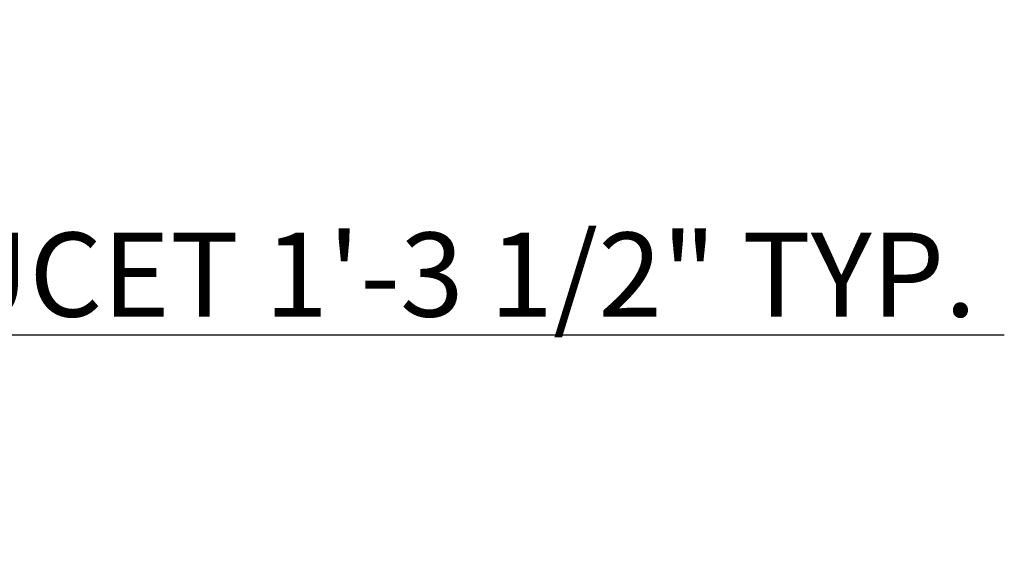
# Model space of a CAD drawing. Units: inches. Extents: x 3064 to 19385, y 846 to 15425.
# Tile 25 of 108: x 3992 to 4098, y 1161 to 1218. Entities that reach past the tile are written whole.
import ezdxf

# ---------------------------------------------------------------- set-up
doc = ezdxf.new("R2010")
doc.units = ezdxf.units.IN
doc.layers.add('A-ANNO-DIMS', color=2, linetype='Continuous', lineweight=18)
doc.styles.get("Standard").update_dxf_attribs({"font": 'arial.ttf'})
doc.dimstyles.new('ISO-25', dxfattribs={"dimtxt": 9, "dimasz": 2.5, "dimexe": 1.25, "dimexo": 0.625, "dimtad": 1, "dimdec": 1, "dimlunit": 3, "dimtxsty": 'Standard', "dimcen": 2.5, "dimadec": 0, "dimazin": 0, "dimtfac": 1, "dimtdec": 1, "dimtmove": 0, "dimatfit": 3, "dimfxl": 1, "dimarcsym": 0})

# ---------------------------------------------------------------- blocks, each defined once
blk = doc.blocks.new('*D407')
at = {"layer": 'A-ANNO-DIMS', "color": 0, "lineweight": -2, "transparency": 16777216}
for p, q in [((3948.96, 1185.71), (3948.96, 1182.73)), ((3964.69, 1185.71), (3964.69, 1182.73)), ((3951.46, 1183.98), (3962.19, 1183.98)), ((3964.69, 1183.98), (4097.55, 1183.98))]:
    blk.add_line(p, q, dxfattribs=at)
at = {"layer": 'A-ANNO-DIMS', "color": 0, "transparency": 16777216}
for points in [[(3951.46, 1184.4), (3951.46, 1183.56), (3948.96, 1183.98)], [(3962.19, 1184.4), (3962.19, 1183.56), (3964.69, 1183.98)]]:
    blk.add_solid(points, dxfattribs=at)
at = {"layer": 'Defpoints', "color": 0, "transparency": 16777216}
for p in [(3948.96, 1186.34), (3964.69, 1186.34), (3964.69, 1183.98)]:
    blk.add_point(p, dxfattribs=at)
at = {"layer": 'A-ANNO-DIMS', "color": 0, "transparency": 16777216, "insert": (4032.37, 1189.26), "char_height": 9, "attachment_point": 5}
blk.add_mtext('FAUCET 1\'-3 1/2" TYP.', dxfattribs=at)

msp = doc.modelspace()

# ---------------------------------------------------------------- dimensions: what is measured, and where the dimension line sits
at = {"layer": 'A-ANNO-DIMS'}
dim = msp.add_linear_dim(base=(3964.69, 1183.98), p1=(3948.96, 1186.34), p2=(3964.69, 1186.34), text='FAUCET <> TYP.', dimstyle='ISO-25', override={"dimdec": 1, "dimrnd": 0, "dimzin": 1, "dimlunit": 4, "dimfrac": 2}, dxfattribs=at)
dim.commit()
dim.dimension.update_dxf_attribs({"geometry": '*D407', "text_midpoint": (4032.37, 1189.26)})

doc.saveas('drawing.dxf')
